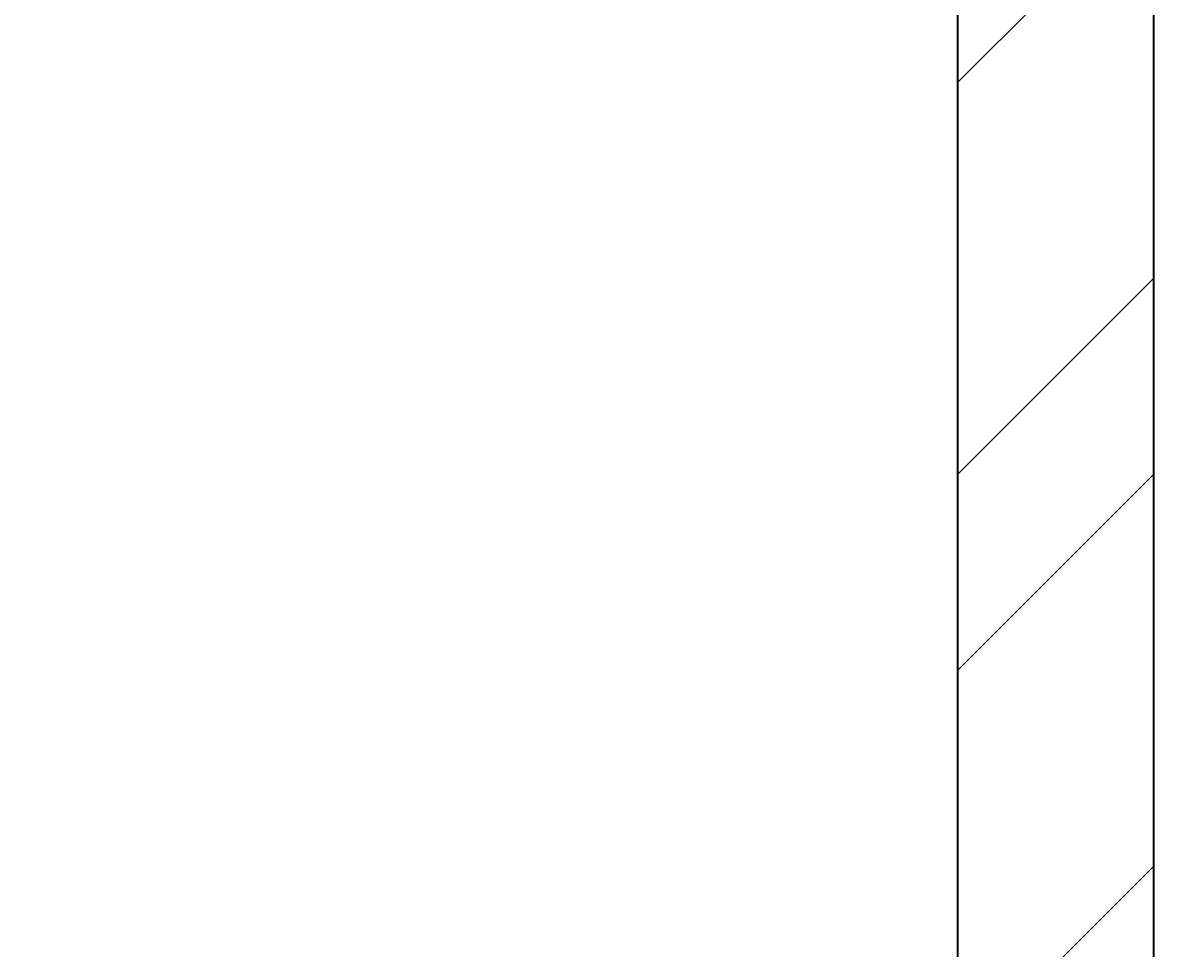
# Model space of a CAD drawing. Units: inches. Extents: x 1885 to 2748, y 783 to 2421.
# Tile 66 of 117: x 1995 to 2022, y 1979 to 2000. Entities that reach past the tile are written whole.
import ezdxf

# ---------------------------------------------------------------- set-up
doc = ezdxf.new("R2010")
doc.units = ezdxf.units.IN
doc.layers.add('A-ANNO-DIMS', color=2, linetype='Continuous', lineweight=18)
doc.layers.add('A-WALL', color=7, linetype='Continuous', lineweight=35)
doc.layers.add('A-WALL-PATT', color=85, linetype='Continuous', lineweight=13, true_color=0x58ba48)
doc.styles.get("Standard").update_dxf_attribs({"font": 'arial.ttf'})
doc.dimstyles.get("Standard").update_dxf_attribs({"dimtxt": 0.18, "dimasz": 0.18, "dimexe": 0.18, "dimexo": 0.0625, "dimgap": 0.09, "dimtad": 0, "dimtih": 1, "dimtoh": 1, "dimdec": 4, "dimzin": 0, "dimdsep": 46, "dimtxsty": 'Standard', "dimcen": 0.09, "dimadec": 0, "dimazin": 0, "dimtfac": 1, "dimtdec": 4, "dimtofl": 0, "dimtmove": 0, "dimatfit": 3, "dimfxl": 1, "dimtolj": 1, "dimtzin": 0, "dimarcsym": 0})

# ---------------------------------------------------------------- blocks, each defined once
blk = doc.blocks.new('*D48')
at = {"layer": 'A-ANNO-DIMS', "color": 0, "lineweight": -2, "transparency": 16777216}
for p, q in [((1980.711, 2348.006), (1902.844, 2348.006)), ((1903.024, 2347.826), (1903.024, 2114.937)), ((1903.024, 1881.686), (1903.024, 2114.574)), ((2016.711, 1881.506), (1902.844, 1881.506))]:
    blk.add_line(p, q, dxfattribs=at)
at = {"layer": 'A-ANNO-DIMS', "color": 0, "transparency": 16777216}
for points in [[(1902.994, 2347.826), (1903.054, 2347.826), (1903.024, 2348.006)], [(1902.994, 1881.686), (1903.054, 1881.686), (1903.024, 1881.506)]]:
    blk.add_solid(points, dxfattribs=at)
at = {"layer": 'Defpoints', "color": 0, "transparency": 16777216}
for p in [(1903.024, 2348.006), (1980.774, 2348.006), (2016.774, 1881.506)]:
    blk.add_point(p, dxfattribs=at)
at = {"layer": 'A-ANNO-DIMS', "color": 0, "transparency": 16777216, "insert": (1903.024, 2114.756), "char_height": 0.18, "attachment_point": 5}
blk.add_mtext('\\A1;466.5', dxfattribs=at)

msp = doc.modelspace()

# ---------------------------------------------------------------- hatches: boundary and pattern name
at = {"layer": 'A-WALL-PATT'}
h = msp.add_hatch(dxfattribs=at)
h.set_pattern_fill('ANSI32', color=256)
h.paths.add_polyline_path([(2007.772, 2318.006), (1980.774, 2318.006), (1980.774, 2281.215), (1985.274, 2281.215), (1985.274, 2313.506), (2007.772, 2313.506), (2007.772, 2315.756)])
h.paths.add_polyline_path([(2094.324, 2318.006), (2067.772, 2318.006), (2067.772, 2313.506), (2094.324, 2313.506), (2094.324, 2315.756)])
h.paths.add_polyline_path([(2131.367, 2315.756), (2131.367, 2318.006), (2131.189, 2318.006), (2112.609, 2318.006), (2112.609, 2313.506), (2117.274, 2313.506), (2117.274, 2255.201), (2121.774, 2255.201), (2121.774, 2313.506), (2131.367, 2313.506)])
h.paths.add_polyline_path([(2190.512, 2318.006), (2155.367, 2318.006), (2155.367, 2313.506), (2169.774, 2313.506), (2169.774, 2229.506), (2121.774, 2229.506), (2121.774, 2233.451), (2119.524, 2233.451), (2117.274, 2233.451), (2117.274, 2201.101), (2121.774, 2201.101), (2121.774, 2225.006), (2169.774, 2225.006), (2169.774, 2165.006), (2306.274, 2165.006), (2306.274, 2066.006), (2310.774, 2066.006), (2344.274, 2066.006), (2486.274, 2066.006), (2486.274, 1886.006), (2483.02, 1886.006), (2483.02, 1881.506), (2486.274, 1881.506), (2486.274, 1880.678), (2490.774, 1880.678), (2490.774, 2070.506), (2344.274, 2070.506), (2310.774, 2070.506), (2310.774, 2165.006), (2310.774, 2173.636), (2308.524, 2173.636), (2306.274, 2173.636), (2306.274, 2169.506), (2174.274, 2169.506), (2174.274, 2313.506), (2190.512, 2313.506), (2190.512, 2315.756)])
h.paths.add_polyline_path([(1985.274, 2221.215), (1980.774, 2221.215), (1980.774, 2165.006), (1992.774, 2165.006), (1992.774, 2141.927), (1997.274, 2141.927), (1997.274, 2165.006), (2117.274, 2165.006), (2117.274, 2163.126), (2121.774, 2163.126), (2121.774, 2172.734), (2119.524, 2172.734), (2117.274, 2172.734), (2117.274, 2169.506), (1985.274, 2169.506)])
h.paths.add_polyline_path([(1997.274, 2105.927), (1992.774, 2105.927), (1992.774, 2070.506), (2016.774, 2070.506), (2016.774, 2059.123), (2019.024, 2059.123), (2021.274, 2059.123), (2021.274, 2070.506), (2117.274, 2070.506), (2117.274, 2022.506), (2114.423, 2022.506), (2114.423, 2018.006), (2123.627, 2018.006), (2123.627, 2020.256), (2123.627, 2022.506), (2121.774, 2022.506), (2121.774, 2142.587), (2119.524, 2142.587), (2117.274, 2142.587), (2117.274, 2075.006), (1997.274, 2075.006)])
h.paths.add_polyline_path([(2092.029, 2020.256), (2092.029, 2022.506), (2021.274, 2022.506), (2021.274, 2035.123), (2016.774, 2035.123), (2016.774, 2018.006), (2016.774, 1978.784), (2021.274, 1978.784), (2021.274, 2018.006), (2092.029, 2018.006)])
h.paths.add_polyline_path([(2260.938, 2022.506), (2153.105, 2022.506), (2153.105, 2020.256), (2153.105, 2018.006), (2155.274, 2018.006), (2155.274, 1886.006), (2107.629, 1886.006), (2107.629, 1881.506), (2182.911, 1881.506), (2182.911, 1883.756), (2182.911, 1886.006), (2159.774, 1886.006), (2159.774, 2018.006), (2260.938, 2018.006), (2260.938, 2020.256)])
h.paths.add_polyline_path([(2047.629, 1883.756), (2047.629, 1886.006), (2021.274, 1886.006), (2021.274, 1918.784), (2019.024, 1918.784), (2016.774, 1918.784), (2016.774, 1881.506), (2047.629, 1881.506)])
h.paths.add_polyline_path([(2306.361, 1883.756), (2306.361, 1886.006), (2296.274, 1886.006), (2296.274, 1982.006), (2316.535, 1982.006), (2316.535, 1984.256), (2316.535, 1986.506), (2296.274, 1986.506), (2296.274, 2022.506), (2289.276, 2022.506), (2289.276, 2018.006), (2291.774, 2018.006), (2291.774, 1886.006), (2242.911, 1886.006), (2242.911, 1881.506), (2306.361, 1881.506)], flags=17)
h.paths.add_polyline_path([(1985.274, 1843.006), (2021.6, 1843.006), (2021.534, 1845.441), (2021.477, 1847.506), (1980.774, 1847.506), (1980.774, 1809.446), (1985.274, 1809.446)])
h.paths.add_polyline_path([(2131.482, 1845.256), (2131.482, 1847.506), (2081.534, 1847.506), (2081.534, 1843.006), (2117.274, 1843.006), (2117.274, 1784.147), (2119.524, 1784.147), (2121.774, 1784.147), (2121.774, 1843.006), (2131.482, 1843.006)])
h.paths.add_polyline_path([(2203.886, 1847.506), (2155.482, 1847.506), (2155.482, 1843.006), (2169.774, 1843.006), (2169.774, 1759.006), (2121.774, 1759.006), (2121.774, 1761.457), (2117.274, 1761.457), (2117.274, 1730.429), (2121.774, 1730.429), (2121.774, 1754.506), (2177.421, 1754.506), (2177.421, 1756.756), (2177.421, 1759.006), (2174.274, 1759.006), (2174.274, 1843.006), (2203.886, 1843.006)])
h.paths.add_polyline_path([(2335.554, 1845.256), (2335.554, 1847.506), (2239.886, 1847.506), (2239.886, 1843.006), (2306.274, 1843.006), (2306.274, 1759.006), (2199.486, 1759.006), (2199.486, 1754.506), (2310.774, 1754.506), (2310.774, 1843.006), (2335.554, 1843.006)])
h.paths.add_polyline_path([(2348.774, 2022.506), (2344.274, 2022.506), (2344.274, 1986.506), (2341.681, 1986.506), (2341.681, 1982.006), (2344.274, 1982.006), (2344.274, 1886.006), (2330.361, 1886.006), (2330.361, 1881.506), (2361.627, 1881.506), (2361.627, 1883.756), (2361.627, 1886.006), (2348.774, 1886.006)], flags=17)
h.paths.add_polyline_path([(2283.251, 2315.756), (2283.251, 2318.006), (2238.512, 2318.006), (2238.512, 2313.506), (2283.251, 2313.506)], flags=17)
h.paths.add_polyline_path([(2363.274, 2348.006), (2388.677, 2348.006), (2388.677, 2350.256), (2388.677, 2352.506), (2358.774, 2352.506), (2358.774, 2348.006), (2358.774, 2318.006), (2344.481, 2318.006), (2344.481, 2313.506), (2358.774, 2313.506), (2358.774, 2229.506), (2310.774, 2229.506), (2310.774, 2231.952), (2306.274, 2231.952), (2306.274, 2205.611), (2310.774, 2205.611), (2310.774, 2225.006), (2358.774, 2225.006), (2358.774, 2211.506), (2452.329, 2211.506), (2452.329, 2213.756), (2452.329, 2216.006), (2363.274, 2216.006), (2363.274, 2318.006)])
h.paths.add_polyline_path([(2310.774, 2313.506), (2320.481, 2313.506), (2320.481, 2315.756), (2320.481, 2318.006), (2302.728, 2318.006), (2302.728, 2313.506), (2306.274, 2313.506), (2306.274, 2251.076), (2310.774, 2251.076)], flags=17)
h.paths.add_polyline_path([(2490.774, 2352.506), (2486.274, 2352.506), (2448.677, 2352.506), (2448.677, 2348.006), (2486.274, 2348.006), (2486.274, 2318.006), (2486.274, 2216.006), (2481.78, 2216.006), (2481.78, 2211.506), (2486.274, 2211.506), (2486.274, 2165.006), (2493.289, 2165.006), (2493.289, 2167.256), (2493.289, 2169.506), (2490.774, 2169.506), (2490.774, 2313.506), (2494.429, 2313.506), (2494.429, 2318.006), (2490.774, 2318.006)])
h.paths.add_polyline_path([(2534.653, 2318.006), (2515.691, 2318.006), (2515.691, 2313.506), (2534.653, 2313.506), (2534.653, 2315.756)])
h.paths.add_polyline_path([(2618.274, 2318.006), (2594.653, 2318.006), (2594.653, 2313.506), (2613.774, 2313.506), (2613.774, 2281.706), (2618.274, 2281.706)])
h.paths.add_polyline_path([(2618.274, 2221.706), (2613.774, 2221.706), (2613.774, 2169.506), (2554.019, 2169.506), (2554.019, 2165.006), (2613.774, 2165.006), (2613.774, 2152.878), (2618.274, 2152.878)])
h.paths.add_polyline_path([(2618.274, 2128.878), (2616.024, 2128.878), (2613.774, 2128.878), (2613.774, 2117.006), (2529.774, 2117.006), (2529.774, 2165.006), (2532.848, 2165.006), (2532.848, 2169.506), (2522.867, 2169.506), (2522.867, 2165.006), (2525.274, 2165.006), (2525.274, 2117.006), (2525.274, 2112.506), (2525.274, 2108.576), (2529.774, 2108.576), (2529.774, 2112.506), (2613.774, 2112.506), (2613.774, 2080.19), (2618.274, 2080.19)])
h.paths.add_polyline_path([(2618.274, 2044.19), (2616.024, 2044.19), (2613.774, 2044.19), (2613.774, 2015.506), (2529.774, 2015.506), (2529.774, 2088.582), (2527.524, 2088.582), (2525.274, 2088.582), (2525.274, 2011.006), (2613.774, 2011.006), (2613.774, 1956.755), (2618.274, 1956.755)])
h.paths.add_polyline_path([(2618.274, 1881.506), (2618.274, 1896.755), (2613.774, 1896.755), (2613.774, 1881.506), (2613.774, 1847.506), (2592.715, 1847.506), (2592.715, 1843.006), (2613.774, 1843.006), (2613.774, 1765.006), (2613.774, 1760.506), (2609.621, 1760.506), (2609.621, 1756.006), (2613.774, 1756.006), (2613.774, 1660.006), (2608.544, 1660.006), (2608.544, 1655.506), (2613.774, 1655.506), (2613.774, 1508.158), (2618.274, 1508.158)])
h.paths.add_polyline_path([(2565.774, 1843.006), (2568.997, 1843.006), (2568.997, 1847.506), (2490.774, 1847.506), (2490.774, 1849.7), (2488.524, 1849.7), (2486.274, 1849.7), (2486.274, 1847.506), (2477.274, 1847.506), (2477.274, 1838.506), (2477.274, 1821.493), (2486.274, 1821.493), (2486.274, 1838.506), (2561.274, 1838.506), (2561.274, 1765.006), (2486.274, 1765.006), (2486.274, 1786.157), (2477.274, 1786.157), (2477.274, 1765.006), (2477.274, 1756.006), (2486.274, 1756.006), (2565.774, 1756.006), (2585.621, 1756.006), (2585.621, 1758.256), (2585.621, 1760.506), (2565.774, 1760.506), (2565.774, 1765.006)])
h.paths.add_polyline_path([(2486.274, 1651.006), (2561.274, 1651.006), (2561.274, 1567.006), (2486.274, 1567.006), (2486.274, 1591.321), (2477.274, 1591.321), (2477.274, 1567.006), (2477.274, 1558.006), (2477.274, 1555.439), (2481.774, 1555.439), (2481.774, 1558.006), (2568.653, 1558.006), (2568.653, 1560.256), (2568.653, 1562.506), (2565.774, 1562.506), (2565.774, 1655.506), (2584.544, 1655.506), (2584.544, 1657.756), (2584.544, 1660.006), (2565.774, 1660.006), (2486.274, 1660.006), (2477.274, 1660.006), (2477.274, 1651.006), (2477.274, 1632.989), (2486.274, 1632.989)])
h.paths.add_polyline_path([(2449.967, 1883.756), (2449.967, 1886.006), (2421.627, 1886.006), (2421.627, 1881.506), (2449.967, 1881.506)], flags=17)
h.paths.add_polyline_path([(2447.274, 1847.506), (2395.554, 1847.506), (2395.554, 1843.006), (2442.774, 1843.006), (2442.774, 1809.27), (2447.274, 1809.27)])
h.paths.add_polyline_path([(1985.274, 1749.446), (1980.774, 1749.446), (1980.774, 1694.504), (1985.274, 1694.504), (1985.274, 1694.506), (1986.897, 1694.506), (1986.897, 1697.78), (1986.897, 1699.006), (1985.274, 1699.006)])
h.paths.add_polyline_path([(2152.774, 1699.006), (2121.774, 1699.006), (2121.774, 1703.668), (2119.524, 1703.668), (2117.274, 1703.668), (2117.274, 1699.006), (2009.219, 1699.006), (2009.219, 1694.506), (2148.274, 1694.506), (2148.274, 1692.631), (2152.774, 1692.631)])
h.paths.add_polyline_path([(2016.274, 1694.506), (2011.774, 1694.506), (2011.774, 1558.006), (2040.806, 1558.006), (2040.806, 1560.256), (2040.806, 1562.506), (2016.274, 1562.506)])
h.paths.add_polyline_path([(2152.774, 1663.017), (2150.524, 1663.017), (2148.274, 1663.017), (2148.274, 1562.506), (2100.806, 1562.506), (2100.806, 1558.006), (2165.119, 1558.006), (2165.119, 1560.256), (2165.119, 1562.506), (2152.774, 1562.506), (2152.774, 1610.506), (2224.774, 1610.506), (2224.774, 1607.99), (2229.274, 1607.99), (2229.274, 1615.006), (2152.774, 1615.006)])
h.paths.add_polyline_path([(2238.613, 1560.256), (2238.613, 1562.506), (2229.274, 1562.506), (2229.274, 1588.756), (2227.024, 1588.763), (2224.774, 1588.771), (2224.774, 1562.506), (2189.119, 1562.506), (2189.119, 1558.006), (2238.613, 1558.006)])
h.paths.add_polyline_path([(2336.024, 1560.256), (2336.024, 1562.506), (2310.774, 1562.506), (2310.774, 1656.347), (2308.524, 1656.347), (2306.274, 1656.347), (2306.274, 1562.506), (2286.613, 1562.506), (2286.613, 1558.006), (2336.024, 1558.006)])
h.paths.add_polyline_path([(2447.274, 1690.968), (2445.024, 1690.968), (2442.774, 1690.968), (2442.774, 1687.006), (2306.274, 1687.006), (2306.274, 1680.75), (2310.774, 1680.75), (2310.774, 1682.506), (2442.774, 1682.506), (2442.774, 1562.506), (2396.024, 1562.506), (2396.024, 1558.006), (2447.274, 1558.006)])
h.paths.add_polyline_path([(2447.274, 1749.27), (2445.024, 1749.27), (2442.774, 1749.27), (2442.774, 1717.232), (2447.274, 1717.232)])
h.paths.add_polyline_path([(2044.674, 1521.756), (2044.674, 1524.006), (2007.274, 1524.006), (2007.274, 1503.49), (2009.524, 1503.49), (2011.774, 1503.49), (2011.774, 1519.506), (2044.674, 1519.506)])
h.paths.add_polyline_path([(2177.969, 1521.756), (2177.969, 1524.006), (2104.674, 1524.006), (2104.674, 1519.506), (2145.774, 1519.506), (2145.774, 1387.506), (2143.37, 1387.506), (2143.37, 1383.006), (2251.585, 1383.006), (2251.585, 1385.256), (2251.585, 1387.506), (2150.274, 1387.506), (2150.274, 1519.506), (2177.969, 1519.506)])
h.paths.add_polyline_path([(2298.704, 1524.006), (2237.969, 1524.006), (2237.969, 1519.506), (2282.274, 1519.506), (2282.274, 1387.506), (2279.683, 1387.506), (2279.683, 1383.006), (2286.774, 1383.006), (2286.774, 1419.006), (2312.451, 1419.006), (2312.451, 1421.256), (2312.451, 1423.506), (2286.774, 1423.506), (2286.774, 1519.506), (2298.704, 1519.506), (2298.704, 1521.722)], flags=17)
h.paths.add_polyline_path([(2361.897, 1521.756), (2361.897, 1524.006), (2322.704, 1524.006), (2322.704, 1519.506), (2334.774, 1519.506), (2334.774, 1423.506), (2331.93, 1423.506), (2331.93, 1419.006), (2334.774, 1419.006), (2334.774, 1387.506), (2334.774, 1383.228), (2339.274, 1383.228), (2339.274, 1387.506), (2339.274, 1519.506), (2361.897, 1519.506)], flags=17)
h.paths.add_polyline_path([(2447.274, 1521.756), (2447.274, 1524.006), (2421.897, 1524.006), (2421.897, 1519.506), (2447.274, 1519.506)], flags=17)
h.paths.add_polyline_path([(2481.774, 1529.6), (2479.524, 1529.6), (2477.274, 1529.6), (2477.274, 1524.006), (2474.489, 1524.006), (2474.489, 1519.506), (2477.274, 1519.506), (2477.274, 1334.506), (2296.774, 1334.506), (2296.774, 1240.506), (2160.274, 1240.506), (2160.274, 1180.506), (2112.274, 1180.506), (2112.274, 1207.692), (2110.024, 1207.692), (2107.774, 1207.692), (2107.774, 1171.609), (2112.274, 1171.609), (2112.274, 1176.006), (2160.274, 1176.006), (2160.274, 1092.006), (2144.221, 1092.006), (2144.221, 1087.506), (2189.497, 1087.506), (2189.497, 1089.756), (2189.497, 1092.006), (2164.774, 1092.006), (2164.774, 1236.006), (2296.774, 1236.006), (2296.774, 1231.912), (2301.274, 1231.912), (2301.274, 1330.006), (2481.774, 1330.006), (2481.774, 1387.506)])
h.paths.add_polyline_path([(2618.274, 1448.158), (2613.774, 1448.158), (2613.774, 1382.506), (2529.774, 1382.506), (2525.274, 1382.506), (2525.274, 1307.062), (2529.774, 1307.062), (2529.774, 1378.006), (2613.774, 1378.006), (2613.774, 1354.988), (2618.274, 1354.988)])
h.paths.add_polyline_path([(2618.274, 1318.988), (2613.774, 1318.988), (2613.774, 1281.006), (2529.774, 1281.006), (2529.774, 1283.786), (2527.524, 1283.786), (2525.274, 1283.786), (2525.274, 1228.506), (2516.794, 1228.506), (2516.794, 1224.006), (2533.484, 1224.006), (2533.484, 1226.256), (2533.484, 1228.506), (2529.774, 1228.506), (2529.774, 1276.506), (2613.774, 1276.506), (2613.774, 1266.02), (2618.274, 1266.02)])
h.paths.add_polyline_path([(2618.274, 1134.964), (2613.774, 1134.964), (2613.774, 1092.006), (2594.545, 1092.006), (2594.545, 1087.506), (2618.274, 1087.506)])
h.paths.add_polyline_path([(2534.545, 1092.006), (2509.765, 1092.006), (2509.765, 1087.506), (2534.545, 1087.506), (2534.545, 1089.756)])
h.paths.add_polyline_path([(2481.274, 1224.006), (2484.117, 1224.006), (2484.117, 1226.256), (2484.117, 1228.506), (2476.774, 1228.506), (2476.774, 1198.506), (2471.61, 1198.506), (2471.61, 1194.006), (2476.774, 1194.006), (2476.774, 1062.006), (2436.894, 1062.006), (2436.894, 1057.506), (2476.774, 1057.506), (2481.274, 1057.506), (2481.274, 1062.006), (2481.274, 1087.506), (2485.354, 1087.506), (2485.354, 1089.756), (2485.354, 1092.006), (2481.274, 1092.006), (2481.274, 1117.506)])
h.paths.add_polyline_path([(2439.898, 1198.506), (2349.274, 1198.506), (2349.274, 1194.006), (2349.274, 1180.506), (2301.274, 1180.506), (2301.274, 1201.896), (2299.024, 1201.896), (2296.774, 1201.896), (2296.774, 1172.335), (2299.024, 1172.335), (2301.274, 1172.335), (2301.274, 1176.006), (2349.274, 1176.006), (2349.274, 1092.006), (2334.452, 1092.006), (2334.452, 1087.506), (2349.274, 1087.506), (2349.274, 1057.506), (2353.774, 1057.506), (2376.894, 1057.506), (2376.894, 1059.756), (2376.894, 1062.006), (2353.774, 1062.006), (2353.774, 1087.506), (2353.774, 1180.506), (2353.774, 1194.006), (2439.898, 1194.006), (2439.898, 1196.256)])
h.paths.add_polyline_path([(2270.596, 1089.756), (2270.596, 1092.006), (2249.497, 1092.006), (2249.497, 1087.506), (2270.596, 1087.506)], flags=17)
h.paths.add_polyline_path([(2310.452, 1092.006), (2301.274, 1092.006), (2301.274, 1153.292), (2296.774, 1153.292), (2296.774, 1092.006), (2293.786, 1092.006), (2293.786, 1087.506), (2310.452, 1087.506), (2310.452, 1089.756)], flags=17)
h.paths.add_polyline_path([(2112.274, 1150.328), (2110.024, 1150.328), (2107.774, 1150.328), (2107.774, 1092.006), (2104.465, 1092.006), (2104.465, 1087.506), (2120.221, 1087.506), (2120.221, 1089.756), (2120.221, 1092.006), (2112.274, 1092.006)])
h.paths.add_polyline_path([(2082.172, 1092.006), (2058.144, 1092.006), (2058.144, 1087.506), (2082.172, 1087.506), (2082.172, 1089.756)])
h.paths.add_polyline_path([(1975.774, 1145.638), (1971.274, 1145.638), (1971.274, 1087.506), (1980.774, 1087.506), (1998.144, 1087.506), (1998.144, 1089.756), (1998.144, 1092.006), (1985.274, 1092.006), (1975.774, 1092.006)])
h.paths.add_polyline_path([(2112.274, 1244.385), (2110.024, 1244.385), (2107.774, 1244.385), (2107.774, 1240.506), (1992.274, 1240.506), (1992.274, 1271.008), (1987.774, 1271.008), (1987.774, 1240.506), (1980.774, 1240.506), (1975.774, 1240.506), (1971.274, 1240.506), (1971.274, 1205.638), (1975.774, 1205.638), (1975.774, 1236.006), (2107.774, 1236.006), (2107.774, 1233.444), (2112.274, 1233.444), (2112.274, 1236.006)])
h.paths.add_polyline_path([(2112.274, 1383.006), (2114.783, 1383.006), (2114.783, 1385.256), (2114.783, 1387.506), (2102.476, 1387.506), (2102.476, 1383.006), (2107.774, 1383.006), (2107.774, 1335.006), (2011.774, 1335.006), (2011.774, 1349.939), (2007.274, 1349.939), (2007.274, 1335.006), (1987.774, 1335.006), (1987.774, 1330.506), (1987.774, 1307.008), (1992.274, 1307.008), (1992.274, 1330.506), (2007.274, 1330.506), (2107.774, 1330.506), (2107.774, 1264.711), (2112.274, 1264.711)])
h.paths.add_polyline_path([(2077.857, 1387.506), (2011.774, 1387.506), (2011.774, 1390.036), (2009.524, 1390.036), (2007.274, 1390.036), (2007.274, 1373.939), (2011.774, 1373.939), (2011.774, 1383.006), (2077.857, 1383.006)])
h.paths.add_polyline_path([(2011.774, 1443.49), (2007.274, 1443.49), (2007.274, 1410.248), (2011.774, 1410.248)])

# ---------------------------------------------------------------- linework, layer by layer
at = {"layer": 'A-WALL'}
for p, q in [((2016.774, 2018.006), (2016.774, 1978.784)), ((2021.274, 1978.784), (2021.274, 2018.006))]:
    msp.add_line(p, q, dxfattribs=at)

# ---------------------------------------------------------------- dimensions: what is measured, and where the dimension line sits
at = {"layer": 'A-ANNO-DIMS'}
dim = msp.add_linear_dim(base=(1903.024, 2348.006), p1=(2016.774, 1881.506), p2=(1980.774, 2348.006), angle=90, dimstyle='Standard', override={"dimdec": 1, "dimlfac": 1, "dimrnd": 0, "dimzin": 0, "dimdsep": 46, "dimlunit": 2}, dxfattribs=at)
dim.commit()
dim.dimension.update_dxf_attribs({"geometry": '*D48', "text_midpoint": (1903.024, 2114.756)})

doc.saveas('drawing.dxf')
